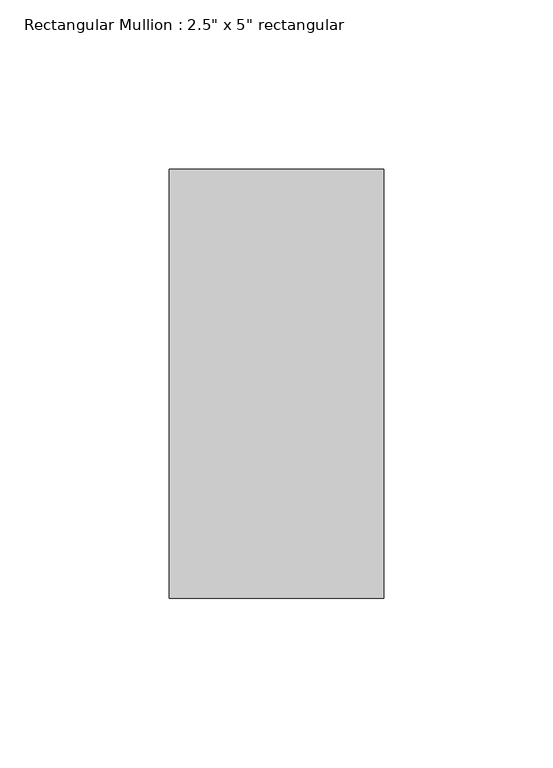
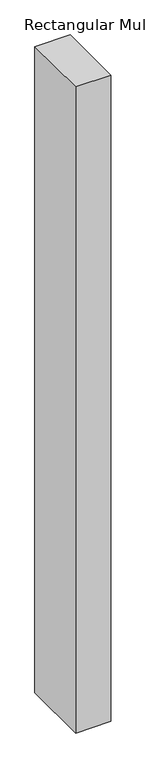
"""IFC4 building model written with IfcOpenShell, lengths in millimetres: member geometry."""

from ifc_helpers import new_model, si_unit, frame, origin, place, context, project, spatial, polyline, outline, extrude, source, transform, mapped, element, save


def member_49503176(model_context):
    return source(origin(), model_context, "Body", "SweptSolid", [
        extrude(outline(polyline([(0.0, 63.5), (0.0, -63.5), (-63.5, -63.5), (-63.5, 63.5), (0.0, 63.5)])), frame((0.0, 0.0, -1231.9), z_axis=(0.0, 0.0, 1.0), x_axis=(1.0, 0.0, 0.0)), (0.0, 0.0, 1.0), 1231.9),
    ])


if __name__ == "__main__":
    model = new_model("IFC4")
    model_context = context("Model", 3, world=origin())
    ifc_project = project(units=[si_unit("LENGTHUNIT", "METRE", prefix="MILLI")], contexts=[model_context])
    site = spatial("IfcSite", under=ifc_project)
    building = spatial("IfcBuilding", under=site)
    placement = place(None, origin())
    member_shape = member_49503176(model_context)
    element("IfcMember", 1, ObjectType="Rectangular Mullion : 2.5\" x 5\" rectangular", at=placement, inside=building, context=model_context, shape_type="MappedRepresentation", body=[
        mapped(member_shape, transform((0.0, 0.0, 0.0), x_axis=(1.0, 0.0, 0.0), y_axis=(0.0, 1.0, 0.0), z_axis=(0.0, 0.0, 1.0))),
    ])
    save(model, "model.ifc")

# Revit data of these elements
# Type "Rectangular Mullion : 2.5\" x 5\" rectangular"
#   built-in parameter 1007304 = 0.416667 (stored number, unit not read)
#   built-in parameter 1007301 = 0.104167 (stored number, unit not read)
#   built-in parameter 1007300 = 0.104167 (stored number, unit not read)
# Element 1 (IfcMember, "Rectangular Mullion : 2.5\" x 5\" rectangular")
#   Materials on its faces: "Aluminum"
# Materials
#   "Aluminum": class "Metal", colour RGB 247 247 247, transparency 0, Description = "Aluminum 6061", Cost = 0
